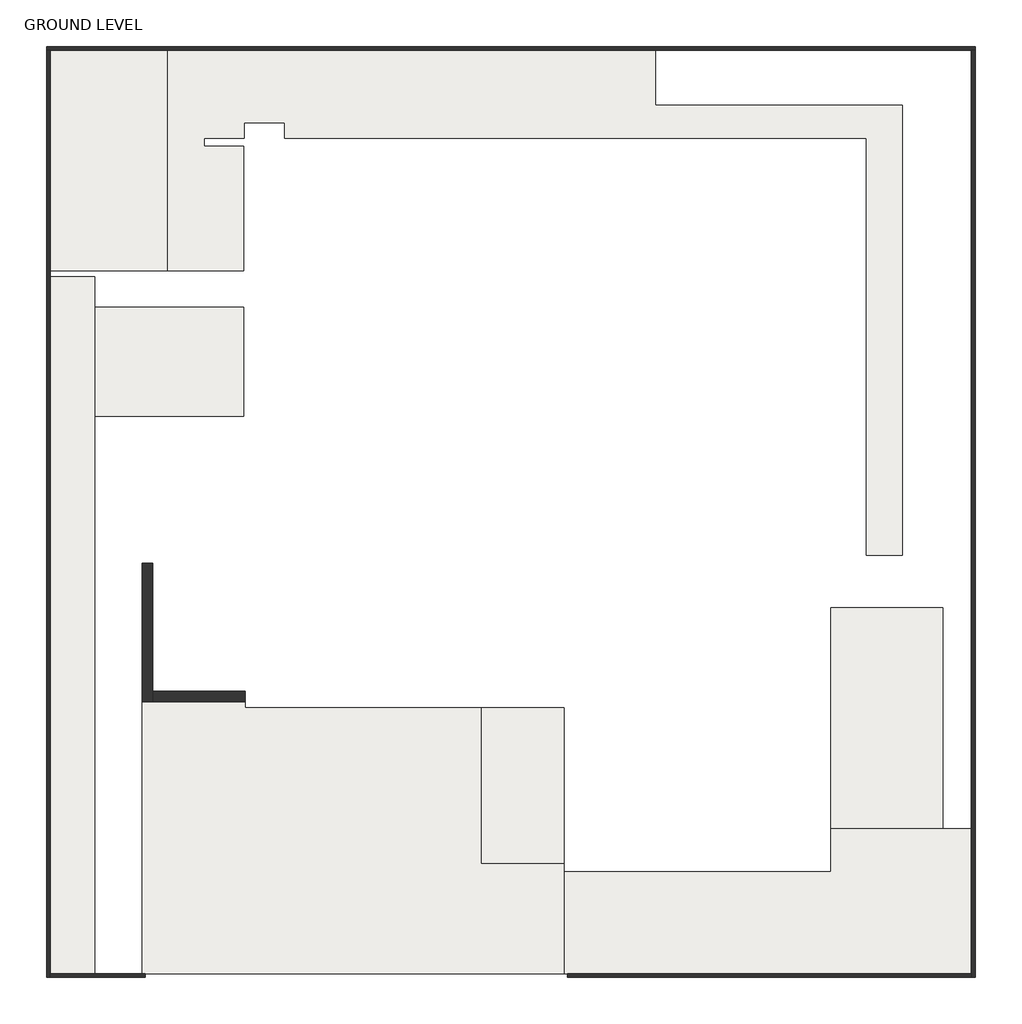
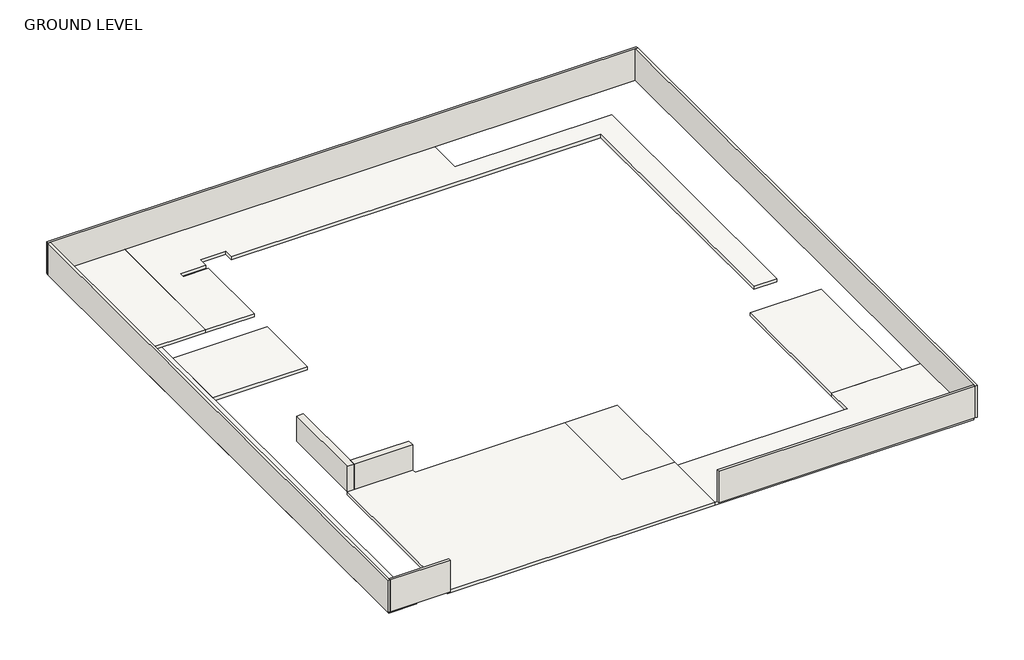
# One storey: 8 slabs, 7 walls.
"""IFC4 building model written with IfcOpenShell, lengths in millimetres."""

from ifc_helpers import new_model, si_unit, frame, origin, origin_with_axes, place, context, project, spatial, polyline, outline, extrude, faceted_brep, element, save

model = new_model("IFC4")

# Units and contexts
model_context = context("Model", 3, world=origin())
ifc_project = project(units=[si_unit("LENGTHUNIT", "METRE", prefix="MILLI")], contexts=[model_context])

# Site, building, storey
site = spatial("IfcSite", under=ifc_project)
building = spatial("IfcBuilding", under=site)
storey = spatial("IfcBuildingStorey", under=building, Name="GROUND LEVEL", Elevation=0.0)

# Slabs
placement = place(None, origin())
element("IfcSlab", 1, at=placement, inside=storey, context=model_context, shape_type="SweptSolid", body=[
    extrude(outline(polyline([(-5592.644009, 12719.9097639), (-7813.1954918, 12719.9097639), (-7813.1954918, 19100.6394725), (6334.6045082, 19100.6394725), (6334.6045082, 17508.432458), (13497.4045082, 17508.432458), (13497.4045082, 4478.232458), (12443.3045082, 4478.232458), (12443.3045082, 16558.8375339), (-4417.894009, 16558.8375339), (-4417.894009, 17000.8847206), (-5577.3305586, 17000.8847206), (-5577.3305586, 16556.19348), (-6748.344009, 16556.19348), (-6748.344009, 16327.59348), (-5592.644009, 16327.59348), (-5592.644009, 12719.9097639)])), frame((0.0, 0.0, -152.4), z_axis=(0.0, 0.0, 1.0), x_axis=(1.0, 0.0, 0.0)), (0.0, 0.0, 1.0), 152.4),
])
element("IfcSlab", 2, at=placement, inside=storey, context=model_context, shape_type="SweptSolid", body=[
    extrude(outline(polyline([(11418.4558511, -4684.1941378), (11418.4558511, -3436.657798), (15484.9042698, -3436.657798), (15484.9042698, -7636.0724221), (3680.2542698, -7636.0724221), (3680.2542698, -4684.1941378), (11418.4558511, -4684.1941378)])), frame((0.0, 0.0, -152.4), z_axis=(0.0, 0.0, 1.0), x_axis=(1.0, 0.0, 0.0)), (0.0, 0.0, 1.0), 152.4),
])
element("IfcSlab", 3, at=placement, inside=storey, context=model_context, shape_type="SweptSolid", body=[
    extrude(outline(polyline([(3680.2542698, -7636.0724221), (-8539.6262442, -7636.0724221), (-8539.6262442, 247.1216143), (-5555.1262442, 247.1216143), (-5555.1262442, 56.6216143), (1281.336242, 56.6216143), (1281.336242, -4456.1321454), (3680.2542698, -4456.1321454), (3680.2542698, -7636.0724221)])), frame((0.0, 0.0, -152.4), z_axis=(0.0, 0.0, 1.0), x_axis=(1.0, 0.0, 0.0)), (0.0, 0.0, 1.0), 152.4),
])
element("IfcSlab", 4, at=placement, inside=storey, context=model_context, shape_type="SweptSolid", body=[
    extrude(outline(polyline([(-11196.5093583, 12548.4597639), (-9911.9908689, 12548.4597639), (-9911.9908689, 8504.39348), (-9911.9908689, -7636.0724221), (-11196.5093583, -7636.0724221), (-11196.5093583, 12548.4597639)])), frame((0.0, 0.0, -152.4), z_axis=(0.0, 0.0, 1.0), x_axis=(1.0, 0.0, 0.0)), (0.0, 0.0, 1.0), 152.4),
])
element("IfcSlab", 5, ObjectType="METAL DECK FLOORING 6\"", at=placement, inside=storey, context=model_context, shape_type="SweptSolid", body=[
    extrude(outline(polyline([(-5592.644009, 11667.286866), (-5592.644009, 8504.39348), (-9911.9908689, 8504.39348), (-9911.9908689, 11667.286866), (-5592.644009, 11667.286866)])), frame((0.0, 0.0, -152.4), z_axis=(0.0, 0.0, 1.0), x_axis=(1.0, 0.0, 0.0)), (0.0, 0.0, 1.0), 152.4),
])
element("IfcSlab", 6, ObjectType="METAL DECK FLOORING 6\"", at=placement, inside=storey, context=model_context, shape_type="SweptSolid", body=[
    extrude(outline(polyline([(14665.2141504, 2964.142202), (14665.2141504, -3436.657798), (11414.0141504, -3436.657798), (11414.0141504, 2964.142202), (14665.2141504, 2964.142202)])), frame((0.0, 0.0, -152.4), z_axis=(0.0, 0.0, 1.0), x_axis=(1.0, 0.0, 0.0)), (0.0, 0.0, 1.0), 152.4),
])
element("IfcSlab", 7, ObjectType="SITE FLOORING 6\"", at=placement, inside=storey, context=model_context, shape_type="SweptSolid", body=[
    extrude(outline(polyline([(-7813.1954918, 19100.6394725), (-7813.1954918, 12719.9097639), (-11196.5093583, 12719.9097639), (-11196.5093583, 19100.6394725), (-7813.1954918, 19100.6394725)])), frame((0.0, 0.0, -152.4), z_axis=(0.0, 0.0, 1.0), x_axis=(1.0, 0.0, 0.0)), (0.0, 0.0, 1.0), 152.4),
])
element("IfcSlab", 8, ObjectType="SITE FLOORING 6\"", at=placement, inside=storey, context=model_context, shape_type="SweptSolid", body=[
    extrude(outline(polyline([(3679.0904479, 56.6216143), (3679.0904479, -4456.1321454), (1281.336242, -4456.1321454), (1281.336242, 56.6216143), (3679.0904479, 56.6216143)])), frame((0.0, 0.0, -152.4), z_axis=(0.0, 0.0, 1.0), x_axis=(1.0, 0.0, 0.0)), (0.0, 0.0, 1.0), 152.4),
])

# Walls
element("IfcWall", 9, ObjectType="INNER WALL 4.5\"", at=placement, inside=storey, context=model_context, shape_type="Brep", body=[
    faceted_brep([(-11310.8093583, 19100.6394725, 0.0), (-11196.5093583, 19100.6394725, 0.0), (15484.9042698, 19100.6394725, 0.0), (15599.2042698, 19100.6394725, 0.0), (15599.2042698, 19100.6394725, 1524.0), (15484.9042698, 19100.6394725, 1524.0), (-11196.5093583, 19100.6394725, 1524.0), (-11310.8093583, 19100.6394725, 1524.0), (-11310.8093583, 19214.9394725, 0.0), (-11310.8093583, 19214.9394725, 1524.0), (15599.2042698, 19214.9394725, 1524.0), (15599.2042698, 19214.9394725, 0.0)], [[[0, 1, 2, 3, 4, 5, 6, 7]], [[8, 9, 10, 11]], [[3, 2, 1, 0, 8, 11]], [[7, 6, 5, 4, 10, 9]], [[4, 3, 11, 10]], [[0, 7, 9, 8]]]),
])
element("IfcWall", 10, ObjectType="INNER WALL 4.5\"", at=placement, inside=storey, context=model_context, shape_type="Brep", body=[
    faceted_brep([(15484.9042698, 19100.6394725, 0.0), (15484.9042698, -7636.0724221, 0.0), (15484.9042698, -7750.3724221, 0.0), (15484.9042698, -7750.3724221, 1524.0), (15484.9042698, -7636.0724221, 1524.0), (15484.9042698, 19100.6394725, 1524.0), (15599.2042698, 19100.6394725, 0.0), (15599.2042698, 19100.6394725, 1524.0), (15599.2042698, -7750.3724221, 1524.0), (15599.2042698, -7750.3724221, 0.0)], [[[0, 1, 2, 3, 4, 5]], [[6, 7, 8, 9]], [[2, 1, 0, 6, 9]], [[5, 4, 3, 8, 7]], [[0, 5, 7, 6]], [[3, 2, 9, 8]]]),
])
element("IfcWall", 11, ObjectType="INNER WALL 4.5\"", at=placement, inside=storey, context=model_context, shape_type="SweptSolid", body=[
    extrude(outline(polyline([(3782.9367729, -7636.0724221), (15484.9042698, -7636.0724221), (15484.9042698, -7750.3724221), (3782.9367729, -7750.3724221), (3782.9367729, -7636.0724221)])), origin_with_axes(), (0.0, 0.0, 1.0), 1524.0),
])
element("IfcWall", 12, ObjectType="INNER WALL 4.5\"", at=placement, inside=storey, context=model_context, shape_type="Brep", body=[
    faceted_brep([(-11196.5093583, -7750.3724221, 0.0), (-11196.5093583, -7636.0724221, 0.0), (-11196.5093583, 19100.6394725, 0.0), (-11196.5093583, 19100.6394725, 1524.0), (-11196.5093583, -7636.0724221, 1524.0), (-11196.5093583, -7750.3724221, 1524.0), (-11310.8093583, -7750.3724221, 0.0), (-11310.8093583, -7750.3724221, 1524.0), (-11310.8093583, 19100.6394725, 1524.0), (-11310.8093583, 19100.6394725, 0.0)], [[[0, 1, 2, 3, 4, 5]], [[6, 7, 8, 9]], [[2, 1, 0, 6, 9]], [[5, 4, 3, 8, 7]], [[3, 2, 9, 8]], [[0, 5, 7, 6]]]),
])
element("IfcWall", 13, ObjectType="INNER WALL 4.5\"", at=placement, inside=storey, context=model_context, shape_type="SweptSolid", body=[
    extrude(outline(polyline([(-8453.3093583, -7750.3724221), (-11196.5093583, -7750.3724221), (-11196.5093583, -7636.0724221), (-8453.3093583, -7636.0724221), (-8453.3093583, -7750.3724221)])), origin_with_axes(), (0.0, 0.0, 1.0), 1524.0),
])
element("IfcWall", 14, ObjectType="WALL THICKNESS 1'", at=placement, inside=storey, context=model_context, shape_type="Brep", body=[
    faceted_brep([(-8533.2762442, 4247.6216143, 0.0), (-8533.2762442, 241.696878, 0.0), (-8533.2762442, 241.696878, 1219.2), (-8533.2762442, 4247.6216143, 1219.2), (-8533.2762442, 4247.6216143, 304.8), (-8228.4762442, 4247.6216143, 0.0), (-8228.4762442, 4247.6216143, 1219.2), (-8228.4762442, 546.496878, 1219.2), (-8228.4762442, 241.696878, 1219.2), (-8228.4762442, 241.696878, 0.0), (-8228.4762442, 546.496878, 0.0)], [[[0, 1, 2, 3, 4]], [[5, 6, 7, 8, 9, 10]], [[1, 0, 5, 10, 9]], [[3, 2, 8, 7, 6]], [[0, 4, 3, 6, 5]], [[2, 1, 9, 8]]]),
])
element("IfcWall", 15, ObjectType="WALL THICKNESS 1'", at=placement, inside=storey, context=model_context, shape_type="SweptSolid", body=[
    extrude(outline(polyline([(-8228.4762442, 546.496878), (-5555.1262442, 546.496878), (-5555.1262442, 241.696878), (-8228.4762442, 241.696878), (-8228.4762442, 546.496878)])), origin_with_axes(), (0.0, 0.0, 1.0), 1219.2),
])

save(model, "model.ifc")

# Revit data of these elements
# Type
#   Assembly Code = "B1010"
#   Function = 0
#   Layers, outside or top first: 0' - 6" "Grass" (function 1)
# Type
#   Assembly Code = "B1010"
#   Function = 0
# Type "METAL DECK FLOORING 6\""
#   Assembly Code = "B1010"
#   Function = 0
#   Layers, outside or top first: 0' - 6" "WOODEN DECK" (function 1)
# Type "SITE FLOORING 6\""
#   Assembly Code = "B1010"
#   Function = 0
#   Layers, outside or top first: 0' - 6" "SITE FLOORING" (function 1)
# Type "INNER WALL 4.5\""
#   Assembly Code = "B2010"
#   Layers, outside or top first: 0' - 4 1/2" "BEIGE COLOUR" (function 1)
# Type "WALL THICKNESS 1'"
#   Assembly Code = "B2010"
#   Layers, outside or top first: 1' - 0" "BEIGE COLOUR" (function 1)
# Elements 1, 2 (IfcSlab)
#   Height Offset From Level = 0' - 0"
#   Phase Created = New Construction
#   Materials on its faces: "Grass"
# Element 3 (IfcSlab)
#   Height Offset From Level = 0' - 0"
#   Phase Created = New Construction
# Element 4 (IfcSlab)
#   built-in parameter 1001955 = 3.14159 (stored number, unit not read)
#   Height Offset From Level = 0' - 0"
#   Phase Created = New Construction
# Elements 5, 6 (IfcSlab, "METAL DECK FLOORING 6\"")
#   Height Offset From Level = 0' - 0"
#   Phase Created = New Construction
#   Materials on its faces: "WOODEN DECK"
# Elements 7, 8 (IfcSlab, "SITE FLOORING 6\"")
#   Height Offset From Level = 0' - 0"
#   Phase Created = New Construction
#   Materials on its faces: "SITE FLOORING"
# Elements 9, 10, 11, 12, 13 (IfcWall, "INNER WALL 4.5\"")
#   Top Offset = 0' - 0"
#   Base Offset = 0' - 0"
#   Unconnected Height = 5' - 0"
#   wall height = 5' - 0"
#   Phase Created = New Construction
#   Base Constraint = GROUND LEVEL
#   Materials on its faces: "BEIGE COLOUR"
# Elements 14, 15 (IfcWall, "WALL THICKNESS 1'")
#   Top Offset = 0' - 0"
#   Base Offset = 0' - 0"
#   Unconnected Height = 4' - 0"
#   wall height = 4' - 0"
#   Phase Created = New Construction
#   Base Constraint = GROUND LEVEL
#   Materials on its faces: "BEIGE COLOUR"
# Materials
#   "Grass": class "Generic", colour RGB 104 137 66, transparency 0, Description = "Physical material.", Cost = 0
#   "WOODEN DECK": class "Generic", colour RGB 120 120 120, transparency 0, Cost = 0
#   "SITE FLOORING": class "Generic", colour RGB 120 120 120, transparency 0, Cost = 0
#   "BEIGE COLOUR": class "Generic", colour RGB 120 120 120, transparency 0, Cost = 0
